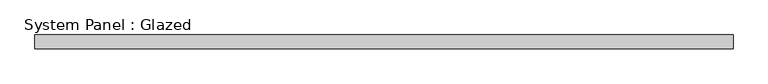
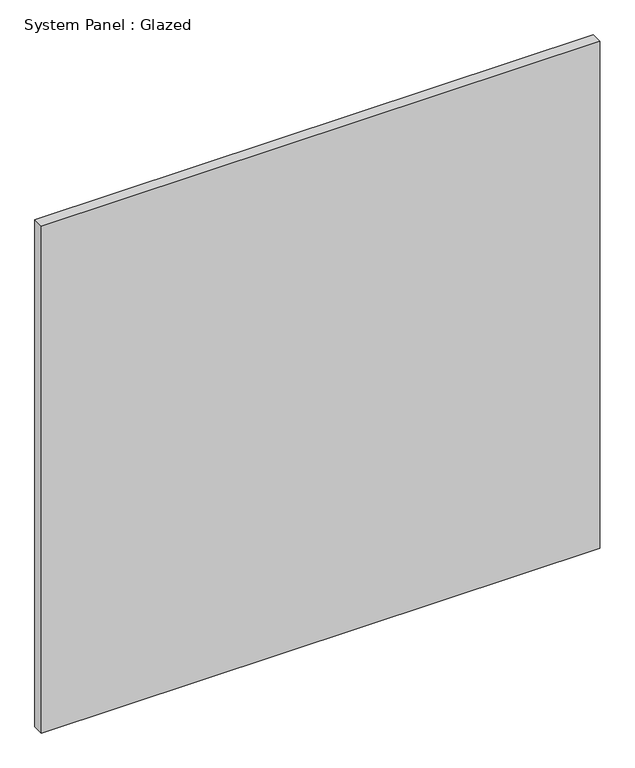
"""IFC4 building model written with IfcOpenShell, lengths in millimetres: plate geometry, System Panel : Glazed."""

from ifc_helpers import new_model, si_unit, origin, origin_with_axes, place, context, project, spatial, polyline, outline, extrude, source, transform, mapped, element, save


def system_panel_glazed_729cd57b(model_context):
    return source(origin(), model_context, "Body", "SweptSolid", [
        extrude(outline(polyline([(635.0, 19.05), (-635.0, 19.05), (-635.0, 44.45), (635.0, 44.45), (635.0, 19.05)])), origin_with_axes(), (0.0, 0.0, 1.0), 1219.2),
    ])


if __name__ == "__main__":
    model = new_model("IFC4")
    model_context = context("Model", 3, world=origin())
    ifc_project = project(units=[si_unit("LENGTHUNIT", "METRE", prefix="MILLI")], contexts=[model_context])
    site = spatial("IfcSite", under=ifc_project)
    building = spatial("IfcBuilding", under=site)
    placement = place(None, origin())
    system_panel_glazed_shape = system_panel_glazed_729cd57b(model_context)
    element("IfcPlate", 1, ObjectType="System Panel : Glazed", at=placement, inside=building, context=model_context, shape_type="MappedRepresentation", body=[
        mapped(system_panel_glazed_shape, transform((0.0, 0.0, 0.0), x_axis=(1.0, 0.0, 0.0), y_axis=(0.0, 1.0, 0.0), z_axis=(0.0, 0.0, 1.0))),
    ])
    save(model, "model.ifc")

# Revit data of these elements
# Type "System Panel : Glazed"
#   Construction Type Id = "GSP4R"
#   Analytic Construction = "1/8 in Pilkington single glazing"
#   Visual Light Transmittance = 0.9
#   Solar Heat Gain Coefficient = 0.86
#   Heat Transfer Coefficient (U) = 1.18115 BTU/(h·ft²·°F)
# Element 1 (IfcPlate, "System Panel : Glazed")
#   Materials on its faces: "Glass"
# Materials
#   "Glass": class "Glass", colour RGB 0 128 192, transparency 0.75, Description = "Soda Lime Glass", Cost = 0
